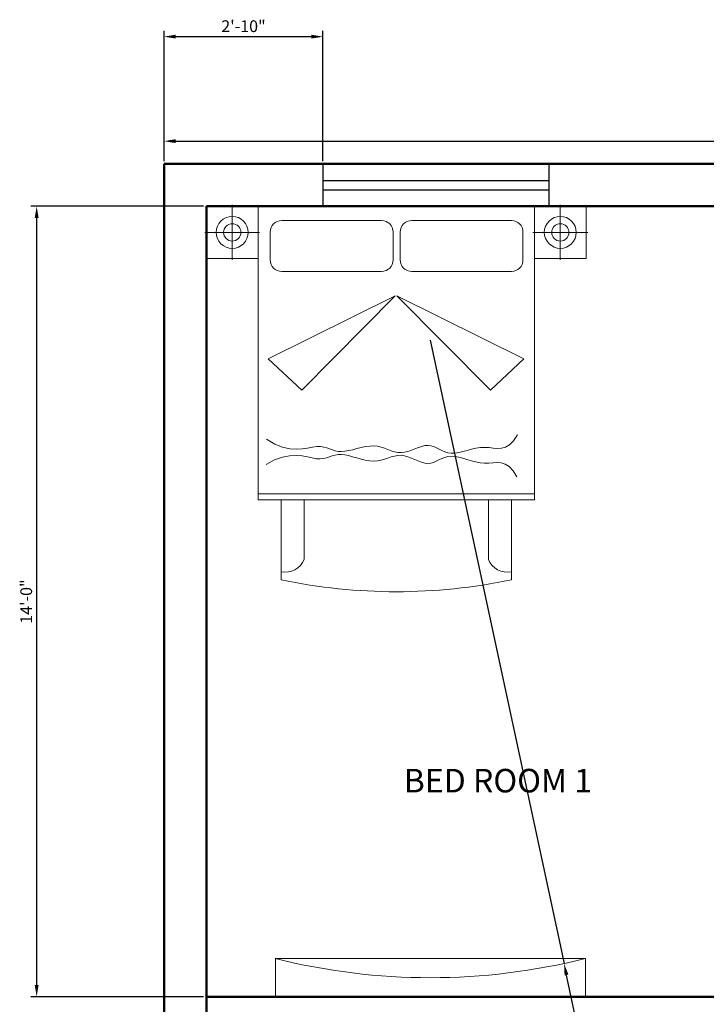
# Model space of a CAD drawing. Units: inches. Extents: x 1905 to 2315, y 3232 to 3824.
# Tile 6 of 8: x 1907 to 2053, y 3615 to 3824. Entities that reach past the tile are written whole.
import ezdxf

# ---------------------------------------------------------------- set-up
doc = ezdxf.new("R2010")
doc.units = ezdxf.units.IN
for name, color, linetype, lineweight in [('A-ANNO-DIMS', 2, 'Continuous', 18), ('A-AREA-IDEN', 7, 'Continuous', 25), ('A-FURN', 8, 'Continuous', 18), ('TV', 221, 'Continuous', 18), ('wall', 2, 'Continuous', 50), ('WINDOW', 60, 'Continuous', 25)]:
    doc.layers.add(name, color=color, linetype=linetype, lineweight=lineweight)
doc.styles.get("Standard").update_dxf_attribs({"font": 'arial.ttf'})
doc.dimstyles.new('ISO-25', dxfattribs={"dimtxt": 2.5, "dimasz": 2.5, "dimexe": 1.25, "dimexo": 0.625, "dimtad": 1, "dimdec": 1, "dimlunit": 3, "dimtxsty": 'Standard', "dimcen": 2.5, "dimadec": 0, "dimazin": 0, "dimtfac": 1, "dimtdec": 1, "dimtmove": 0, "dimatfit": 3, "dimfxl": 1, "dimarcsym": 0})

# ---------------------------------------------------------------- blocks, each defined once
blk = doc.blocks.new('A$C4F543DC7')
for p, q in [((0.0134, 3.35, -0.1688), (3.3134, 3.35, -0.1688)), ((0.4634, 3.35, -0.1688), (0.0134, 3.35, -0.1688)), ((0.0134, 2.896, -0.1688), (0.0134, 3.35, -0.1688)), ((0.0134, 3.35, -0.1688), (0.0134, 2.896, -0.1688)), ((0.2381, 3.1233, -0.4388), (0.2381, 3.3614, -0.4388)), ((0.4634, 3.35, -0.1688), (0.4634, 0.8, -0.1688)), ((2.8634, 3.35, -0.1688), (0.4634, 3.35, -0.1688)), ((0.4634, 2.896, -0.1688), (0.4634, 3.35, -0.1688)), ((2.8634, 0.8, -0.1688), (2.8634, 3.35, -0.1688)), ((2.8634, 3.35, -0.1688), (3.3134, 3.35, -0.1688)), ((2.8634, 2.896, -0.1688), (2.8634, 3.35, -0.1688)), ((3.0888, 3.1233, -0.4388), (3.0888, 3.3614, -0.4388)), ((3.3134, 3.35, -0.1688), (3.3134, 2.896, -0.1688)), ((3.3134, 3.35, -0.1688), (3.3134, 2.896, -0.1688)), ((1.5354, 3.226, -0.1688), (0.6684, 3.226, -0.1688)), ((2.6644, 3.226, -0.1688), (1.7974, 3.226, -0.1688)), ((0.2381, 3.1233, -0.4388), (0, 3.1233, -0.4388)), ((0.2381, 3.1233, -0.4388), (0.4762, 3.1233, -0.4388)), ((0.2381, 3.1233, -0.4388), (0.2381, 2.8852, -0.4388)), ((0.5684, 3.126, -0.1688), (0.5684, 2.884, -0.1688)), ((1.6354, 2.884, -0.1688), (1.6354, 3.126, -0.1688)), ((1.6974, 3.126, -0.1688), (1.6974, 2.884, -0.1688)), ((2.7644, 2.884, -0.1688), (2.7644, 3.126, -0.1688)), ((3.0888, 3.1233, -0.4388), (2.8507, 3.1233, -0.4388)), ((3.0888, 3.1233, -0.4388), (3.0888, 2.8852, -0.4388)), ((3.0888, 3.1233, -0.4388), (3.3269, 3.1233, -0.4388)), ((0.4634, 2.896, -0.1688), (0.0134, 2.896, -0.1688)), ((0.0134, 2.896, -0.1688), (0.4634, 2.896, -0.1688)), ((0.4634, 0.8, -0.1688), (0.4634, 2.896, -0.1688)), ((2.8634, 2.896, -0.1688), (2.8634, 0.8, -0.1688)), ((3.3134, 2.896, -0.1688), (2.8634, 2.896, -0.1688)), ((3.3134, 2.896, -0.1688), (2.8634, 2.896, -0.1688)), ((0.6684, 2.784, -0.1688), (1.5354, 2.784, -0.1688)), ((1.7974, 2.784, -0.1688), (2.6644, 2.784, -0.1688)), ((1.6534, 2.573, -0.1688), (0.5504, 2.025, -0.1688)), ((0.8414, 1.752, -0.1688), (1.6534, 2.573, -0.1688)), ((2.4814, 1.752, -0.1688), (1.6694, 2.573, -0.1688)), ((1.6694, 2.573, -0.1688), (2.7724, 2.025, -0.1688)), ((0.5504, 2.025, -0.1688), (0.8414, 1.752, -0.1688)), ((2.7724, 2.025, -0.1688), (2.4814, 1.752, -0.1688)), ((0.5369, 1.3267, -0.1688), (0.6088, 1.2835, -0.1688)), ((2.6479, 1.2774, -0.1688), (2.683, 1.312, -0.1688)), ((2.683, 1.312, -0.1688), (2.7182, 1.3641, -0.1688)), ((0.6088, 1.2835, -0.1688), (0.6756, 1.2566, -0.1688)), ((0.6756, 1.2566, -0.1688), (0.7373, 1.2428, -0.1688)), ((0.7373, 1.2428, -0.1688), (0.794, 1.239, -0.1688)), ((0.794, 1.239, -0.1688), (0.8457, 1.242, -0.1688)), ((0.8457, 1.242, -0.1688), (0.8925, 1.2489, -0.1688)), ((0.8925, 1.2489, -0.1688), (0.9345, 1.2564, -0.1688)), ((0.9345, 1.2564, -0.1688), (0.9718, 1.2615, -0.1688)), ((0.9718, 1.2615, -0.1688), (1.0044, 1.2617, -0.1688)), ((1.0044, 1.2617, -0.1688), (1.0334, 1.2578, -0.1688)), ((1.0334, 1.2578, -0.1688), (1.0597, 1.2509, -0.1688)), ((1.0597, 1.2509, -0.1688), (1.0842, 1.2424, -0.1688)), ((1.0842, 1.2424, -0.1688), (1.1081, 1.2336, -0.1688)), ((1.1081, 1.2336, -0.1688), (1.1322, 1.2257, -0.1688)), ((1.1322, 1.2257, -0.1688), (1.1577, 1.2201, -0.1688)), ((1.1577, 1.2201, -0.1688), (1.1855, 1.218, -0.1688)), ((1.1855, 1.218, -0.1688), (1.2163, 1.2204, -0.1688)), ((1.2163, 1.2204, -0.1688), (1.2498, 1.2264, -0.1688)), ((1.2498, 1.2264, -0.1688), (1.2852, 1.2347, -0.1688)), ((1.2852, 1.2347, -0.1688), (1.3218, 1.2441, -0.1688)), ((1.3218, 1.2441, -0.1688), (1.3591, 1.2533, -0.1688)), ((1.3591, 1.2533, -0.1688), (1.3963, 1.2612, -0.1688)), ((1.3963, 1.2612, -0.1688), (1.4328, 1.2664, -0.1688)), ((1.4328, 1.2664, -0.1688), (1.4679, 1.2677, -0.1688)), ((1.4679, 1.2677, -0.1688), (1.501, 1.2643, -0.1688)), ((1.501, 1.2643, -0.1688), (1.5324, 1.257, -0.1688)), ((1.5324, 1.257, -0.1688), (1.5624, 1.2473, -0.1688)), ((1.5624, 1.2473, -0.1688), (1.5915, 1.2365, -0.1688)), ((1.5915, 1.2365, -0.1688), (1.6199, 1.2259, -0.1688)), ((1.6199, 1.2259, -0.1688), (1.6481, 1.2169, -0.1688)), ((1.6481, 1.2169, -0.1688), (1.6765, 1.2108, -0.1688)), ((1.6765, 1.2108, -0.1688), (1.7053, 1.209, -0.1688)), ((1.7053, 1.209, -0.1688), (1.7349, 1.2124, -0.1688)), ((1.7349, 1.2124, -0.1688), (1.7651, 1.2199, -0.1688)), ((1.7651, 1.2199, -0.1688), (1.7955, 1.2301, -0.1688)), ((1.7955, 1.2301, -0.1688), (1.8258, 1.2417, -0.1688)), ((1.8258, 1.2417, -0.1688), (1.8557, 1.2531, -0.1688)), ((1.8557, 1.2531, -0.1688), (1.8849, 1.263, -0.1688)), ((1.8849, 1.263, -0.1688), (1.913, 1.2698, -0.1688)), ((1.913, 1.2698, -0.1688), (1.9397, 1.2722, -0.1688)), ((1.9397, 1.2722, -0.1688), (1.9649, 1.2692, -0.1688)), ((1.9649, 1.2692, -0.1688), (1.989, 1.2617, -0.1688)), ((1.989, 1.2617, -0.1688), (2.0124, 1.2512, -0.1688)), ((2.0124, 1.2512, -0.1688), (2.0359, 1.2391, -0.1688)), ((2.0359, 1.2391, -0.1688), (2.0599, 1.2269, -0.1688)), ((2.0599, 1.2269, -0.1688), (2.0849, 1.216, -0.1688)), ((2.0849, 1.216, -0.1688), (2.1117, 1.2077, -0.1688)), ((2.1117, 1.2077, -0.1688), (2.1407, 1.2037, -0.1688)), ((2.1407, 1.2037, -0.1688), (2.1723, 1.2047, -0.1688)), ((2.1723, 1.2047, -0.1688), (2.2062, 1.21, -0.1688)), ((2.2062, 1.21, -0.1688), (2.242, 1.2182, -0.1688)), ((2.242, 1.2182, -0.1688), (2.2791, 1.2279, -0.1688)), ((2.2791, 1.2279, -0.1688), (2.3173, 1.2378, -0.1688)), ((2.3173, 1.2378, -0.1688), (2.3558, 1.2465, -0.1688)), ((2.3558, 1.2465, -0.1688), (2.3944, 1.2527, -0.1688)), ((2.3944, 1.2527, -0.1688), (2.4325, 1.255, -0.1688)), ((2.4325, 1.255, -0.1688), (2.4698, 1.2529, -0.1688)), ((2.4698, 1.2529, -0.1688), (2.5064, 1.2488, -0.1688)), ((2.5064, 1.2488, -0.1688), (2.5423, 1.2459, -0.1688)), ((2.5423, 1.2459, -0.1688), (2.5777, 1.2476, -0.1688)), ((2.5777, 1.2476, -0.1688), (2.6129, 1.257, -0.1688)), ((2.6129, 1.257, -0.1688), (2.6479, 1.2774, -0.1688)), ((0.5334, 1.105, -0.1688), (0.6067, 1.1458, -0.1688)), ((0.6067, 1.1458, -0.1688), (0.6743, 1.1706, -0.1688)), ((0.6743, 1.1706, -0.1688), (0.7364, 1.1825, -0.1688)), ((0.7364, 1.1825, -0.1688), (0.7931, 1.1846, -0.1688)), ((0.7931, 1.1846, -0.1688), (0.8447, 1.1799, -0.1688)), ((0.8447, 1.1799, -0.1688), (0.8913, 1.1716, -0.1688)), ((0.8913, 1.1716, -0.1688), (0.9331, 1.1628, -0.1688)), ((0.9331, 1.1628, -0.1688), (0.9701, 1.1565, -0.1688)), ((0.9701, 1.1565, -0.1688), (1.0027, 1.1552, -0.1688)), ((1.0027, 1.1552, -0.1688), (1.0318, 1.1582, -0.1688)), ((1.0318, 1.1582, -0.1688), (1.0583, 1.1642, -0.1688)), ((1.0583, 1.1642, -0.1688), (1.0831, 1.172, -0.1688)), ((1.0831, 1.172, -0.1688), (1.1072, 1.18, -0.1688)), ((1.1072, 1.18, -0.1688), (1.1316, 1.1872, -0.1688)), ((1.1316, 1.1872, -0.1688), (1.1573, 1.192, -0.1688)), ((1.1573, 1.192, -0.1688), (1.1851, 1.1932, -0.1688)), ((1.1851, 1.1932, -0.1688), (1.2158, 1.1898, -0.1688)), ((1.2158, 1.1898, -0.1688), (1.2491, 1.1828, -0.1688)), ((1.2491, 1.1828, -0.1688), (1.2842, 1.1734, -0.1688)), ((1.2842, 1.1734, -0.1688), (1.3206, 1.1629, -0.1688)), ((1.3206, 1.1629, -0.1688), (1.3575, 1.1524, -0.1688)), ((1.3575, 1.1524, -0.1688), (1.3945, 1.1434, -0.1688)), ((1.3945, 1.1434, -0.1688), (1.4308, 1.1371, -0.1688)), ((1.4308, 1.1371, -0.1688), (1.4658, 1.1347, -0.1688)), ((1.4658, 1.1347, -0.1688), (1.499, 1.137, -0.1688)), ((1.499, 1.137, -0.1688), (1.5306, 1.1433, -0.1688)), ((1.5306, 1.1433, -0.1688), (1.5609, 1.152, -0.1688)), ((1.5609, 1.152, -0.1688), (1.5903, 1.1619, -0.1688)), ((1.5903, 1.1619, -0.1688), (1.6191, 1.1716, -0.1688)), ((1.6191, 1.1716, -0.1688), (1.6475, 1.1797, -0.1688)), ((1.6475, 1.1797, -0.1688), (1.676, 1.1849, -0.1688)), ((1.676, 1.1849, -0.1688), (1.7049, 1.1858, -0.1688)), ((1.7049, 1.1858, -0.1688), (1.7344, 1.1816, -0.1688)), ((1.7344, 1.1816, -0.1688), (1.7643, 1.1731, -0.1688)), ((1.7643, 1.1731, -0.1688), (1.7944, 1.1619, -0.1688)), ((1.7944, 1.1619, -0.1688), (1.8244, 1.1494, -0.1688)), ((1.8244, 1.1494, -0.1688), (1.8539, 1.137, -0.1688)), ((1.8539, 1.137, -0.1688), (1.8827, 1.1263, -0.1688)), ((1.8827, 1.1263, -0.1688), (1.9106, 1.1186, -0.1688)), ((1.9106, 1.1186, -0.1688), (1.9373, 1.1153, -0.1688)), ((1.9373, 1.1153, -0.1688), (1.9625, 1.1176, -0.1688)), ((1.9625, 1.1176, -0.1688), (1.9868, 1.1243, -0.1688)), ((1.9868, 1.1243, -0.1688), (2.0106, 1.134, -0.1688)), ((2.0106, 1.134, -0.1688), (2.0344, 1.1454, -0.1688)), ((2.0344, 1.1454, -0.1688), (2.0588, 1.1568, -0.1688)), ((2.0588, 1.1568, -0.1688), (2.0842, 1.167, -0.1688)), ((2.0842, 1.167, -0.1688), (2.1112, 1.1743, -0.1688)), ((2.1112, 1.1743, -0.1688), (2.1403, 1.1775, -0.1688)), ((2.1403, 1.1775, -0.1688), (2.1718, 1.1755, -0.1688)), ((2.1718, 1.1755, -0.1688), (2.2056, 1.1691, -0.1688)), ((2.2056, 1.1691, -0.1688), (2.2411, 1.1598, -0.1688)), ((2.2411, 1.1598, -0.1688), (2.2779, 1.1489, -0.1688)), ((2.2779, 1.1489, -0.1688), (2.3157, 1.1379, -0.1688)), ((2.3157, 1.1379, -0.1688), (2.354, 1.1279, -0.1688)), ((2.354, 1.1279, -0.1688), (2.3923, 1.1205, -0.1688)), ((2.3923, 1.1205, -0.1688), (2.4304, 1.117, -0.1688)), ((2.4304, 1.117, -0.1688), (2.4677, 1.118, -0.1688)), ((2.4677, 1.118, -0.1688), (2.5043, 1.1209, -0.1688)), ((2.5043, 1.1209, -0.1688), (2.5403, 1.1226, -0.1688)), ((2.5403, 1.1226, -0.1688), (2.5757, 1.1199, -0.1688)), ((2.5757, 1.1199, -0.1688), (2.6106, 1.1094, -0.1688)), ((2.6106, 1.1094, -0.1688), (2.645, 1.0879, -0.1688)), ((2.645, 1.0879, -0.1688), (2.6789, 1.0522, -0.1688)), ((2.6789, 1.0522, -0.1688), (2.7124, 0.999, -0.1688)), ((0.4634, 0.85, -0.1688), (2.8634, 0.85, -0.1688)), ((0.4634, 0.8, -0.1688), (2.8634, 0.8, -0.1688)), ((0.6634, 0.8, -0.1688), (0.4634, 0.8, -0.1688)), ((0.6634, 0.8, -0.1688), (2.6634, 0.8, -0.1688)), ((0.6634, 0.104, -0.1688), (0.6634, 0.8, -0.1688)), ((0.6634, 0.104, -0.1688), (0.6634, 0.8, -0.1688)), ((0.8634, 0.281, -0.1688), (0.8634, 0.8, -0.1688)), ((2.4634, 0.8, -0.1688), (2.4634, 0.281, -0.1688)), ((2.8634, 0.8, -0.1688), (2.6634, 0.8, -0.1688)), ((2.6634, 0.8, -0.1688), (2.6634, 0.104, -0.1688)), ((2.6634, 0.8, -0.1688), (2.6634, 0.104, -0.1688))]:
    blk.add_line(p, q)
for centre, radius in [((0.2381, 3.1233, -0.4388), 0.139), ((3.0888, 3.1233, -0.4388), 0.139), ((0.2381, 3.1233, -0.4388), 0.075), ((3.0888, 3.1233, -0.4388), 0.075)]:
    blk.add_circle(centre, radius)
for centre, radius, start, end in [((0.6684, 3.126, -0.1688), 0.1, 90, 180), ((1.5354, 3.126, -0.1688), 0.1, 0, 90), ((1.7974, 3.126, -0.1688), 0.1, 90, 180), ((2.6644, 3.126, -0.1688), 0.1, 0, 90), ((0.6684, 2.884, -0.1688), 0.1, 180, 270), ((1.5354, 2.884, -0.1688), 0.1, 270, 0), ((1.7974, 2.884, -0.1688), 0.1, 180, 270), ((2.6644, 2.884, -0.1688), 0.1, 270, 0), ((0.6994, 0.3472, -0.1688), 0.1769, 258.2616, 338.03196), ((2.6275, 0.3472, -0.1688), 0.1769, 201.96804, 281.7384), ((1.6634, 4.8597, -0.1688), 4.8597, 258.12517, 281.87483), ((1.6634, 4.8597, -0.1688), 4.8597, 258.12517, 281.87483)]:
    blk.add_arc(centre, radius, start, end)
blk = doc.blocks.new('*D15')
at = {"layer": 'A-ANNO-DIMS', "color": 0, "lineweight": -2, "transparency": 16777216}
for p, q in [((1938.01, 3793.86), (1938.01, 3799.33)), ((2286.01, 3793.86), (2286.01, 3799.33)), ((1940.51, 3798.08), (2283.51, 3798.08))]:
    blk.add_line(p, q, dxfattribs=at)
at = {"layer": 'A-ANNO-DIMS', "color": 0, "transparency": 16777216}
for points in [[(1940.51, 3798.5), (1940.51, 3797.67), (1938.01, 3798.08)], [(2283.51, 3798.5), (2283.51, 3797.67), (2286.01, 3798.08)]]:
    blk.add_solid(points, dxfattribs=at)
at = {"layer": 'Defpoints', "color": 0, "transparency": 16777216}
for p in [(2286.01, 3798.08), (1938.01, 3793.23), (2286.01, 3793.23)]:
    blk.add_point(p, dxfattribs=at)
at = {"layer": 'A-ANNO-DIMS', "color": 0, "transparency": 16777216, "insert": (2112.01, 3799.99), "char_height": 2.5, "attachment_point": 5}
blk.add_mtext("29'", dxfattribs=at)
blk = doc.blocks.new('WIN-48IN')
for p, q in [((0, 9), (0, 0)), ((0, 9), (48, 9)), ((48, 9), (48, 0)), ((0, 5.5), (48, 5.5)), ((0, 3.5), (48, 3.5)), ((0, 0), (48, 0))]:
    blk.add_line(p, q)
blk = doc.blocks.new('*D39')
at = {"layer": 'A-ANNO-DIMS', "color": 0, "lineweight": -2, "transparency": 16777216}
for p, q in [((1938.01, 3793.86), (1938.01, 3821.54)), ((1971.78, 3793.86), (1971.78, 3821.54)), ((1940.51, 3820.29), (1969.28, 3820.29))]:
    blk.add_line(p, q, dxfattribs=at)
at = {"layer": 'A-ANNO-DIMS', "color": 0, "transparency": 16777216}
for points in [[(1940.51, 3820.71), (1940.51, 3819.88), (1938.01, 3820.29)], [(1969.28, 3820.71), (1969.28, 3819.88), (1971.78, 3820.29)]]:
    blk.add_solid(points, dxfattribs=at)
at = {"layer": 'Defpoints', "color": 0, "transparency": 16777216}
for p in [(1971.78, 3820.29), (1938.01, 3793.23), (1971.78, 3793.23)]:
    blk.add_point(p, dxfattribs=at)
at = {"layer": 'A-ANNO-DIMS', "color": 0, "transparency": 16777216, "insert": (1954.89, 3822.19), "char_height": 2.5, "attachment_point": 5}
blk.add_mtext('2\'-10"', dxfattribs=at)
blk = doc.blocks.new('*D48')
at = {"layer": 'A-ANNO-DIMS', "color": 0, "lineweight": -2, "transparency": 16777216}
for p, q in [((1946.38, 3784.23), (1909.7, 3784.23)), ((1910.95, 3618.73), (1910.95, 3781.73)), ((1946.38, 3616.23), (1909.7, 3616.23))]:
    blk.add_line(p, q, dxfattribs=at)
at = {"layer": 'A-ANNO-DIMS', "color": 0, "transparency": 16777216}
for points in [[(1910.53, 3781.73), (1911.36, 3781.73), (1910.95, 3784.23)], [(1910.53, 3618.73), (1911.36, 3618.73), (1910.95, 3616.23)]]:
    blk.add_solid(points, dxfattribs=at)
at = {"layer": 'Defpoints', "color": 0, "transparency": 16777216}
for p in [(1910.95, 3784.23), (1947.01, 3784.23), (1947.01, 3616.23)]:
    blk.add_point(p, dxfattribs=at)
at = {"layer": 'A-ANNO-DIMS', "color": 0, "transparency": 16777216, "insert": (1909.05, 3700.23), "char_height": 2.5, "attachment_point": 5, "rotation": 90}
blk.add_mtext('14\'-0"', dxfattribs=at)
blk = doc.blocks.new('*D77')
at = {"layer": 'A-ANNO-DIMS', "color": 0, "lineweight": -2, "transparency": 16777216}
for p, q in [((1994.59, 3755.82), (2023, 3623.3)), ((2041.94, 3534.97), (2023.52, 3620.86))]:
    blk.add_line(p, q, dxfattribs=at)
at = {"layer": 'A-ANNO-DIMS', "color": 0, "transparency": 16777216}
blk.add_solid([(2023.93, 3620.95), (2023.12, 3620.77), (2023, 3623.3)], dxfattribs=at)
at = {"layer": 'Defpoints', "color": 0, "transparency": 16777216}
for p in [(1994.59, 3755.82), (2023, 3623.3)]:
    blk.add_point(p, dxfattribs=at)
at = {"layer": 'A-ANNO-DIMS', "color": 0, "transparency": 16777216, "insert": (2041.92, 3544.2), "char_height": 2.5, "attachment_point": 5, "rotation": 282.0988}
blk.add_mtext('R11\'-3 1/2"', dxfattribs=at)

msp = doc.modelspace()

# ---------------------------------------------------------------- linework, layer by layer
at = {"layer": 'TV'}
msp.add_lwpolyline([(1961.66, 3616.23), (2027.53, 3616.23), (2027.53, 3624.36), (1961.66, 3624.36)], close=True, dxfattribs=at)
msp.add_arc((1994.59, 3755.82), 135.53, 255.9366, 284.0634, dxfattribs=at)
at = {"layer": 'wall'}
for p, q in [((2286.01, 3793.23), (1938.01, 3793.23)), ((1938.01, 3793.23), (1938.01, 3277.23)), ((2277.01, 3784.23), (1947.01, 3784.23)), ((1947.01, 3784.23), (1947.01, 3286.23)), ((2091.01, 3616.23), (1947.01, 3616.23))]:
    msp.add_line(p, q, dxfattribs=at)

# ---------------------------------------------------------------- block references
at = {"layer": 'A-FURN', "xscale": 24.45263891714, "yscale": 24.45263891714, "zscale": 24.45263891714}
msp.add_blockref('A$C4F543DC7', (1946.68, 3702.32, 4.13), dxfattribs=at)
at = {"layer": 'WINDOW'}
msp.add_blockref('WIN-48IN', (1971.78, 3784.23), dxfattribs=at)

# ---------------------------------------------------------------- texts
at = {"layer": 'A-AREA-IDEN', "insert": (1988.93, 3664.67), "char_height": 5, "attachment_point": 1}
msp.add_mtext_dynamic_manual_height_columns('BED ROOM 1', width=56.1502, gutter_width=12.5, heights=[0], dxfattribs=at)

# ---------------------------------------------------------------- dimensions: what is measured, and where the dimension line sits
at = {"layer": 'A-ANNO-DIMS'}
for base, p2, override, picture, middle in [((1971.78, 3820.29), (1971.78, 3793.23), {"dimdec": 1, "dimlfac": 1, "dimrnd": 0, "dimzin": 1, "dimdsep": 46, "dimlunit": 4, "dimfrac": 2}, '*D39', (1954.89, 3822.19)), ((2286.01, 3798.08), (2286.01, 3793.23), {"dimclrd": 0, "dimclre": 0, "dimclrt": 0}, '*D15', (2112.01, 3799.99))]:
    dim = msp.add_linear_dim(base=base, p1=(1938.01, 3793.23), p2=p2, dimstyle='ISO-25', override=override, dxfattribs=at)
    dim.commit()
    dim.dimension.update_dxf_attribs({"geometry": picture, "text_midpoint": middle})
dim = msp.add_linear_dim(base=(1910.95, 3784.23), p1=(1947.01, 3616.23), p2=(1947.01, 3784.23), angle=90, dimstyle='ISO-25', override={"dimdec": 1, "dimlfac": 1, "dimrnd": 0, "dimzin": 1, "dimdsep": 46, "dimlunit": 4, "dimfrac": 2}, dxfattribs=at)
dim.commit()
dim.dimension.update_dxf_attribs({"geometry": '*D48', "text_midpoint": (1909.05, 3700.23)})
dim = msp.add_radius_dim(center=(1994.59, 3755.82), mpoint=(2023, 3623.3), dimstyle='ISO-25', override={"dimdec": 1, "dimlfac": 1, "dimrnd": 0, "dimzin": 1, "dimdsep": 46, "dimlunit": 4, "dimfrac": 2}, dxfattribs=at)
dim.commit()
dim.dimension.update_dxf_attribs({"geometry": '*D77', "text_midpoint": (2040.04, 3543.79), "dimtype": 164})

doc.saveas('drawing.dxf')
